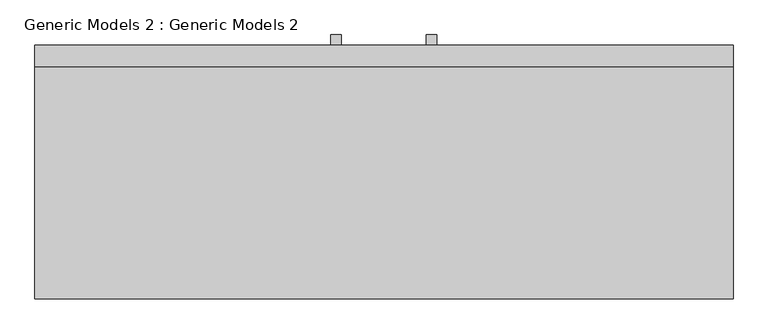
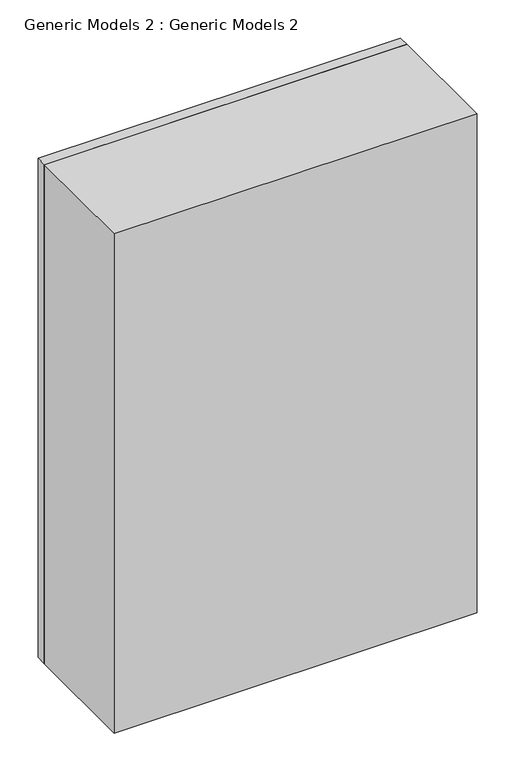
"""IFC4 building model written with IfcOpenShell, lengths in millimetres: proxy geometry, Generic Models 2 : Generic Models 2."""

from ifc_helpers import new_model, si_unit, frame, origin, origin_with_axes, place, context, project, spatial, polyline, outline, extrude, source, transform, mapped, element, save


def generic_models_2_generic_models_2_74e35ba5(model_context):
    return source(origin(), model_context, "Body", "SweptSolid", [
        extrude(outline(polyline([(-2590.2201068, -4006.4122986), (-2564.8201068, -4006.4122986), (-2564.8201068, -4082.6122986), (-2590.2201068, -4082.6122986), (-2590.2201068, -4006.4122986)])), frame((0.0, 0.0, 914.4), z_axis=(0.0, 0.0, 1.0), x_axis=(1.0, 0.0, 0.0)), (0.0, 0.0, 1.0), 609.6),
        extrude(outline(polyline([(-2820.115988, -4006.4122986), (-2794.715988, -4006.4122986), (-2794.715988, -4082.6122986), (-2820.115988, -4082.6122986), (-2820.115988, -4006.4122986)])), frame((0.0, 0.0, 914.4), z_axis=(0.0, 0.0, 1.0), x_axis=(1.0, 0.0, 0.0)), (0.0, 0.0, 1.0), 609.6),
        extrude(outline(polyline([(-2666.4201068, -4031.8122986), (-1891.7201068, -4031.8122986), (-1891.7201068, -4082.6122986), (-2666.4201068, -4082.6122986), (-2666.4201068, -4031.8122986)])), frame((0.0, 0.0, 38.1), z_axis=(0.0, 0.0, 1.0), x_axis=(1.0, 0.0, 0.0)), (0.0, 0.0, 1.0), 2362.2),
        extrude(outline(polyline([(-3491.9201068, -4031.8122986), (-2717.2201068, -4031.8122986), (-2717.2201068, -4082.6122986), (-3491.9201068, -4082.6122986), (-3491.9201068, -4031.8122986)])), frame((0.0, 0.0, 38.1), z_axis=(0.0, 0.0, 1.0), x_axis=(1.0, 0.0, 0.0)), (0.0, 0.0, 1.0), 2362.2),
        extrude(outline(polyline([(2438.4, -3530.0201068), (0.0, -3530.0201068), (0.0, -1853.6201068), (2438.4, -1853.6201068), (2438.4, -3530.0201068)]), holes=[polyline([(2413.0, -2679.1201068), (2413.0, -1879.0201068), (25.4, -1879.0201068), (25.4, -2679.1201068), (2413.0, -2679.1201068)]), polyline([(25.4, -2704.5201068), (25.4, -3504.6201068), (2413.0, -3504.6201068), (2413.0, -2704.5201068), (25.4, -2704.5201068)])]), frame((0.0, -4082.6122986, 0.0), z_axis=(0.0, 1.0, 0.0), x_axis=(0.0, 0.0, 1.0)), (0.0, 0.0, 1.0), 50.8),
        extrude(outline(polyline([(-1853.6201068, -4641.4122986), (-3530.0201068, -4641.4122986), (-3530.0201068, -4082.6122986), (-1853.6201068, -4082.6122986), (-1853.6201068, -4641.4122986)])), origin_with_axes(), (0.0, 0.0, 1.0), 2438.4),
    ])


if __name__ == "__main__":
    model = new_model("IFC4")
    model_context = context("Model", 3, world=origin())
    ifc_project = project(units=[si_unit("LENGTHUNIT", "METRE", prefix="MILLI")], contexts=[model_context])
    site = spatial("IfcSite", under=ifc_project)
    building = spatial("IfcBuilding", under=site)
    placement = place(None, origin())
    generic_models_2_generic_models_2_shape = generic_models_2_generic_models_2_74e35ba5(model_context)
    element("IfcBuildingElementProxy", 1, Name="Generic Models 2 : Generic Models 2", ObjectType="Generic Models 2 : Generic Models 2", at=placement, inside=building, context=model_context, shape_type="MappedRepresentation", body=[
        mapped(generic_models_2_generic_models_2_shape, transform((0.0, 0.0, 0.0), x_axis=(1.0, 0.0, 0.0), y_axis=(0.0, 1.0, 0.0), z_axis=(0.0, 0.0, 1.0))),
    ])
    save(model, "model.ifc")

# Revit data of these elements
# Element 1 (IfcBuildingElementProxy, "Generic Models 2 : Generic Models 2")
#   Materials on its faces: "0 kitchen tiles(3)", "0 kitchen tiles(1)", "0 kitchen tiles(2)"
# Materials
#   "0 kitchen tiles(3)": class "Generic", colour RGB 120 120 120, transparency 0, Cost = 0
#   "0 kitchen tiles(1)": class "Generic", colour RGB 120 120 120, transparency 0, Cost = 0
#   "0 kitchen tiles(2)": class "Generic", colour RGB 120 120 120, transparency 0, Cost = 0
